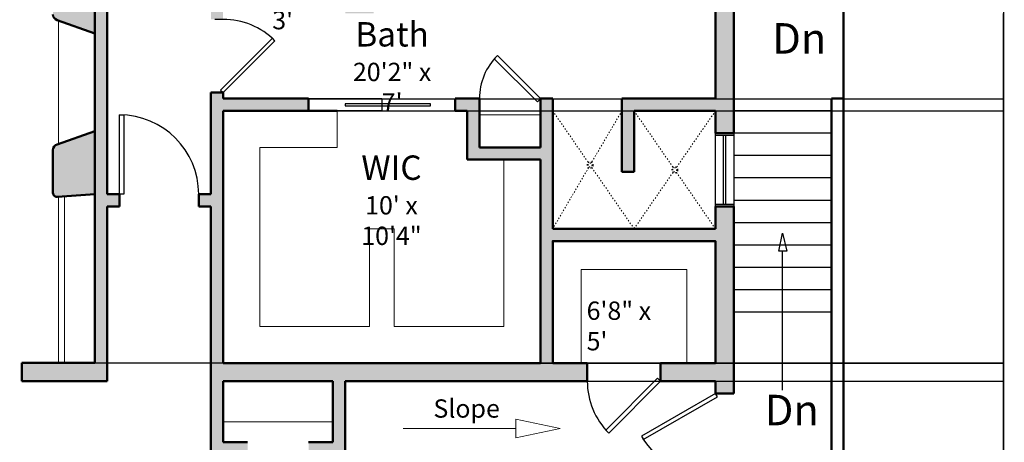
# Model space of a CAD drawing. Units: inches. Extents: x 296 to 2116, y 330 to 1460.
# Tile 4 of 9: x 752 to 1235, y 898 to 1106. Entities that reach past the tile are written whole.
import ezdxf

# ---------------------------------------------------------------- set-up
doc = ezdxf.new("R2010")
doc.units = ezdxf.units.IN
doc.linetypes.add('ACAD_ISO03W100', pattern=[30, 12, -18])
for name, color, linetype, lineweight in [('A-ANNO-DIMS', 2, 'Continuous', 18), ('A-ANNO-SYMB', 2, 'Continuous', 18), ('A-ANNO-TEXT', 7, 'Continuous', 18), ('A-AREA-IDEN', 7, 'Continuous', 25), ('A-DOOR', 3, 'Continuous', 25), ('A-FLOR-FIXT', 8, 'Continuous', 18), ('A-FLOR-OVHD', 132, 'ACAD_ISO03W100', 18), ('A-FLOR-STRS', 40, 'Continuous', 25), ('A-GLAZ', 4, 'Continuous', 25), ('A-WALL', 7, 'Continuous', 50), ('A-WALL-PATT', 8, 'Continuous', 13)]:
    doc.layers.add(name, color=color, linetype=linetype, lineweight=lineweight)
doc.styles.get("Standard").update_dxf_attribs({"font": 'arial.ttf'})
doc.dimstyles.get("Standard").update_dxf_attribs({"dimtxt": 0.18, "dimasz": 0.18, "dimexe": 0.18, "dimexo": 0.0625, "dimgap": 0.09, "dimtad": 0, "dimtih": 1, "dimtoh": 1, "dimdec": 4, "dimzin": 0, "dimdsep": 46, "dimtxsty": 'Standard', "dimcen": 0.09, "dimadec": 0, "dimazin": 0, "dimtfac": 1, "dimtdec": 4, "dimtofl": 0, "dimtmove": 0, "dimatfit": 3, "dimfxl": 1, "dimtolj": 1, "dimtzin": 0, "dimarcsym": 0})

# ---------------------------------------------------------------- blocks, each defined once
blk = doc.blocks.new('*U9')
for p, q in [((0, 0), (0, -4)), ((30, 0), (30, -4))]:
    blk.add_line(p, q)
blk.add_lwpolyline([(0, 0), (21.21, 21.21), (22.45, 19.98), (1.24, -1.24)], close=True)
blk.add_arc((0, 0), 30, 0, 45)
blk = doc.blocks.new('*U11')
for p, q in [((0, 0), (0, -4)), ((-40, 0), (-40, -4))]:
    blk.add_line(p, q)
blk.add_lwpolyline([(0, 0), (-20, 34.64), (-21.52, 33.77), (-1.52, -0.88)], close=True)
blk.add_arc((0, 0), 40, 120, 180)
blk = doc.blocks.new('*U13')
for p, q in [((-32, 0), (-32, 4)), ((0, 0), (0, 4))]:
    blk.add_line(p, q)
blk.add_lwpolyline([(0, 0), (0, -32), (-1.75, -32), (-1.75, 0)], close=True)
blk.add_arc((0, 0), 32, 180, 270)
blk = doc.blocks.new('*U14')
for p, q in [((0, 0), (0, 4)), ((24, 0), (24, 4))]:
    blk.add_line(p, q)
blk.add_lwpolyline([(0, 0), (16.97, -16.97), (18.21, -15.73), (1.24, 1.24)], close=True)
blk.add_arc((0, 0), 24, 315, 0)
blk = doc.blocks.new('*U16')
for p, q in [((0, 0), (0, 4)), ((36, 0), (36, 4))]:
    blk.add_line(p, q)
blk.add_lwpolyline([(0, 0), (25.46, -25.46), (26.69, -24.22), (1.24, 1.24)], close=True)
blk.add_arc((0, 0), 36, 315, 0)
blk = doc.blocks.new('SLOPE-ARROW')
blk.add_line((739.99, 662.71), (684.54, 662.71))
blk.add_lwpolyline([(662.67, 662.71), (684.54, 658.1), (684.54, 667.32)], close=True)
blk = doc.blocks.new('*D45')
at = {"layer": 'A-ANNO-DIMS', "color": 0, "lineweight": -2, "transparency": 16777216}
for p, q in [((1156.58, 1407.95), (1235.3, 1407.95)), ((1235.12, 1407.77), (1235.12, 895.66)), ((1235.12, 383.18), (1235.12, 895.29)), ((609.63, 383), (1235.3, 383))]:
    blk.add_line(p, q, dxfattribs=at)
at = {"layer": 'A-ANNO-DIMS', "color": 0, "transparency": 16777216}
for points in [[(1235.09, 1407.77), (1235.15, 1407.77), (1235.12, 1407.95)], [(1235.09, 383.18), (1235.15, 383.18), (1235.12, 383)]]:
    blk.add_solid(points, dxfattribs=at)
at = {"layer": 'Defpoints', "color": 0, "transparency": 16777216}
for p in [(1156.52, 1407.95), (1235.12, 1407.95), (609.57, 383)]:
    blk.add_point(p, dxfattribs=at)
at = {"layer": 'A-ANNO-DIMS', "color": 0, "transparency": 16777216, "insert": (1235.12, 895.48), "char_height": 0.18, "attachment_point": 5}
blk.add_mtext('\\A1;1025', dxfattribs=at)
blk = doc.blocks.new('*D63')
at = {"layer": 'A-ANNO-DIMS', "color": 0, "lineweight": -2, "transparency": 16777216}
for p, q in [((1102.58, 1156.95), (1235.3, 1156.95)), ((1235.12, 1156.77), (1235.12, 973.64)), ((1235.12, 790.13), (1235.12, 973.27)), ((1063.58, 789.95), (1235.3, 789.95))]:
    blk.add_line(p, q, dxfattribs=at)
at = {"layer": 'A-ANNO-DIMS', "color": 0, "transparency": 16777216}
for points in [[(1235.09, 1156.77), (1235.15, 1156.77), (1235.12, 1156.95)], [(1235.09, 790.13), (1235.15, 790.13), (1235.12, 789.95)]]:
    blk.add_solid(points, dxfattribs=at)
at = {"layer": 'Defpoints', "color": 0, "transparency": 16777216}
for p in [(1102.52, 1156.95), (1235.12, 1156.95), (1063.52, 789.95)]:
    blk.add_point(p, dxfattribs=at)
at = {"layer": 'A-ANNO-DIMS', "color": 0, "transparency": 16777216, "insert": (1235.12, 973.45), "char_height": 0.18, "attachment_point": 5}
blk.add_mtext('\\A1;367', dxfattribs=at)
blk = doc.blocks.new('*D83')
at = {"layer": 'A-ANNO-DIMS', "color": 0, "lineweight": -2, "transparency": 16777216}
for p, q in [((851.58, 1150.95), (1235.3, 1150.95)), ((1235.12, 1150.77), (1235.12, 1109.14)), ((1235.12, 1067.13), (1235.12, 1108.77)), ((851.58, 1066.95), (1235.3, 1066.95))]:
    blk.add_line(p, q, dxfattribs=at)
at = {"layer": 'A-ANNO-DIMS', "color": 0, "transparency": 16777216}
for points in [[(1235.09, 1150.77), (1235.15, 1150.77), (1235.12, 1150.95)], [(1235.09, 1067.13), (1235.15, 1067.13), (1235.12, 1066.95)]]:
    blk.add_solid(points, dxfattribs=at)
at = {"layer": 'Defpoints', "color": 0, "transparency": 16777216}
for p in [(851.52, 1150.95), (1235.12, 1150.95), (851.52, 1066.95)]:
    blk.add_point(p, dxfattribs=at)
at = {"layer": 'A-ANNO-DIMS', "color": 0, "transparency": 16777216, "insert": (1235.12, 1108.95), "char_height": 0.18, "attachment_point": 5}
blk.add_mtext('\\A1;84.00', dxfattribs=at)
blk = doc.blocks.new('*D84')
at = {"layer": 'A-ANNO-DIMS', "color": 0, "lineweight": -2, "transparency": 16777216}
for p, q in [((851.58, 1060.95), (1235.3, 1060.95)), ((1235.12, 1060.77), (1235.12, 999.14)), ((1235.12, 937.13), (1235.12, 998.77)), ((851.58, 936.95), (1235.3, 936.95))]:
    blk.add_line(p, q, dxfattribs=at)
at = {"layer": 'A-ANNO-DIMS', "color": 0, "transparency": 16777216}
for points in [[(1235.09, 1060.77), (1235.15, 1060.77), (1235.12, 1060.95)], [(1235.09, 937.13), (1235.15, 937.13), (1235.12, 936.95)]]:
    blk.add_solid(points, dxfattribs=at)
at = {"layer": 'Defpoints', "color": 0, "transparency": 16777216}
for p in [(851.52, 1060.95), (1235.12, 1060.95), (851.52, 936.95)]:
    blk.add_point(p, dxfattribs=at)
at = {"layer": 'A-ANNO-DIMS', "color": 0, "transparency": 16777216, "insert": (1235.12, 998.95), "char_height": 0.18, "attachment_point": 5}
blk.add_mtext('\\A1;124.00', dxfattribs=at)
blk = doc.blocks.new('*D85')
at = {"layer": 'A-ANNO-DIMS', "color": 0, "lineweight": -2, "transparency": 16777216}
for p, q in [((788.58, 1213), (1235.3, 1213)), ((1235.12, 1212.82), (1235.12, 1075.18)), ((1235.12, 937.18), (1235.12, 1074.82)), ((788.58, 937), (1235.3, 937))]:
    blk.add_line(p, q, dxfattribs=at)
at = {"layer": 'A-ANNO-DIMS', "color": 0, "transparency": 16777216}
for points in [[(1235.09, 1212.82), (1235.15, 1212.82), (1235.12, 1213)], [(1235.09, 937.18), (1235.15, 937.18), (1235.12, 937)]]:
    blk.add_solid(points, dxfattribs=at)
at = {"layer": 'Defpoints', "color": 0, "transparency": 16777216}
for p in [(788.52, 1213), (1235.12, 1213), (788.52, 937)]:
    blk.add_point(p, dxfattribs=at)
at = {"layer": 'A-ANNO-DIMS', "color": 0, "transparency": 16777216, "insert": (1235.12, 1075), "char_height": 0.18, "attachment_point": 5}
blk.add_mtext('\\A1;276.00', dxfattribs=at)
blk = doc.blocks.new('*D98')
at = {"layer": 'A-ANNO-DIMS', "color": 0, "lineweight": -2, "transparency": 16777216}
for p, q in [((1030.58, 927.95), (1235.3, 927.95)), ((1235.12, 927.77), (1235.12, 859.14)), ((1235.12, 790.13), (1235.12, 858.77)), ((1093.58, 789.95), (1235.3, 789.95))]:
    blk.add_line(p, q, dxfattribs=at)
at = {"layer": 'A-ANNO-DIMS', "color": 0, "transparency": 16777216}
for points in [[(1235.09, 927.77), (1235.15, 927.77), (1235.12, 927.95)], [(1235.09, 790.13), (1235.15, 790.13), (1235.12, 789.95)]]:
    blk.add_solid(points, dxfattribs=at)
at = {"layer": 'Defpoints', "color": 0, "transparency": 16777216}
for p in [(1030.52, 927.95), (1235.12, 927.95), (1093.52, 789.95)]:
    blk.add_point(p, dxfattribs=at)
at = {"layer": 'A-ANNO-DIMS', "color": 0, "transparency": 16777216, "insert": (1235.12, 858.95), "char_height": 0.18, "attachment_point": 5}
blk.add_mtext('\\A1;138.00', dxfattribs=at)

msp = doc.modelspace()

# ---------------------------------------------------------------- hatches: boundary and pattern name
at = {"layer": 'A-WALL-PATT'}
h = msp.add_hatch(color=256, dxfattribs=at)
h.dxf.hatch_style = 1
h.paths.add_polyline_path([(656.5723, 927.9991), (668.5723, 927.9991), (668.5723, 936.9991), (650.5723, 936.9991), (650.5723, 897.9991), (356.5223, 897.9991), (356.5223, 955.9991), (347.5223, 955.9991), (347.5223, 888.9991), (423.5723, 888.9991), (423.5723, 766.9991), (432.5723, 766.9991), (432.5723, 834.9991), (453.5723, 834.9991), (468.5723, 834.9991), (468.5723, 840.9991), (432.5723, 840.9991), (432.5723, 888.9991), (504.5723, 888.9991), (504.5723, 840.9991), (504.5723, 834.9991), (531.6223, 834.9991), (531.6223, 768.5344), (527.8443, 764.7564), (530.6728, 761.928), (532.087, 760.5138), (540.5723, 768.9991), (598.0723, 768.9991), (598.0723, 777.9991), (601.8223, 777.9991), (601.8223, 782.1991), (601.8223, 783.9991), (598.0723, 783.9991), (598.0723, 798.9991), (592.0723, 798.9991), (592.0723, 774.9991), (537.6223, 774.9991), (537.6223, 834.9991), (592.0723, 834.9991), (592.0723, 828.9991), (598.0723, 828.9991), (598.0723, 834.9991), (647.5723, 834.9991), (647.5723, 828.9991), (656.5723, 828.9991), (656.5723, 846.9991), (650.5723, 846.9991), (647.5723, 846.9991), (647.5723, 840.9991), (510.5723, 840.9991), (510.5723, 888.9991), (647.5723, 888.9991), (647.5723, 882.9991), (656.5723, 882.9991)])
h.paths.add_polyline_path([(432.5723, 730.9991), (496.5723, 730.9991), (496.5723, 724.9991), (502.5723, 724.9991), (502.5723, 730.9991), (506.6311, 735.058), (502.3885, 739.3006), (500.087, 736.9991), (432.5723, 736.9991), (432.5723, 742.9991), (423.5723, 742.9991), (423.5723, 641.9991), (490.5723, 641.9991), (490.5723, 597.9991), (531.5723, 597.9991), (531.5723, 606.9991), (499.5723, 606.9991), (499.5723, 650.9991), (502.5723, 650.9991), (502.5723, 659.9991), (496.5723, 659.9991), (493.5723, 659.9991), (493.5723, 650.9991), (432.5723, 650.9991)])
h.paths.add_polyline_path([(656.5723, 689.4991), (662.5473, 689.4991), (662.5473, 698.4991), (656.5723, 698.4991), (656.5723, 789.9991), (647.5723, 789.9991), (647.5723, 783.9991), (643.8223, 783.9991), (643.8223, 777.9991), (647.5723, 777.9991), (647.5723, 606.9991), (615.5723, 606.9991), (615.5723, 597.9991), (656.5723, 597.9991)])
h.paths.add_polyline_path([(761.5223, 780.9541), (797.5223, 780.9541), (797.5223, 789.9541), (761.5223, 789.9541), (761.5223, 858.9541), (797.5223, 858.9541), (797.5223, 867.9541), (752.5223, 867.9541), (752.5223, 698.4991), (746.5473, 698.4991), (746.5473, 694.2991), (746.5473, 689.4991), (752.5223, 689.4991), (752.5223, 624.9541), (761.5223, 624.9541)])
h.paths.add_polyline_path([(1102.5223, 795.9541), (1093.5223, 795.9541), (1093.5223, 789.9541), (1063.5223, 789.9541), (881.5223, 789.9541), (881.5223, 837.9541), (911.5223, 837.9541), (911.5223, 849.9541), (907.5223, 849.9541), (905.5223, 849.9541), (905.5223, 843.9541), (845.5223, 843.9541), (845.5223, 834.9541), (849.0223, 834.9541), (851.5223, 834.9541), (851.5223, 837.9541), (875.5223, 837.9541), (875.5223, 789.9541), (851.5223, 789.9541), (851.5223, 792.9541), (845.5223, 792.9541), (845.5223, 789.9541), (833.5223, 789.9541), (833.5223, 785.1541), (833.5223, 780.9541), (1049.5223, 780.9541), (1049.5223, 726.9541), (1053.7223, 726.9541), (1058.5223, 726.9541), (1058.5223, 780.9541), (1102.5223, 780.9541)])
h.paths.add_polyline_path([(761.5223, 588.9541), (752.5223, 588.9541), (752.5223, 564.9541), (761.5223, 564.9541)])
h.paths.add_polyline_path([(809.5223, 480.9541), (761.5223, 480.9541), (761.5223, 528.9541), (752.5223, 528.9541), (752.5223, 471.9541), (809.5223, 471.9541)])
h.paths.add_polyline_path([(1058.5223, 684.9541), (1049.5223, 684.9541), (1049.5223, 480.9541), (1001.5223, 480.9541), (1001.5223, 476.4541), (1001.5223, 471.9541), (1058.5223, 471.9541)])
h.paths.add_polyline_path([(794.5223, 1013.9991), (800.5223, 1013.9991), (800.5223, 1019.9991), (794.5223, 1019.9991), (794.5223, 1296.9541), (785.5223, 1296.9541), (785.5223, 1221.9991), (752.5223, 1221.9991), (752.5223, 1212.9991), (788.5223, 1212.9991), (788.5223, 936.9991), (752.5223, 936.9991), (752.5223, 927.9991), (794.5223, 927.9991)])
h.paths.add_polyline_path([(450.0223, 1191.9991), (398.5223, 1191.9991), (398.5223, 1137.9991), (407.5223, 1137.9991), (407.5223, 1182.9991), (450.0223, 1182.9991)])
h.paths.add_polyline_path([(576.5223, 1212.9991), (612.5223, 1212.9991), (612.5223, 1221.9991), (567.5223, 1221.9991), (567.5223, 1191.9991), (540.0223, 1191.9991), (540.0223, 1182.9991), (576.5223, 1182.9991)])
h.paths.add_polyline_path([(407.5223, 1060.9991), (398.5223, 1060.9991), (398.5223, 1030.9991), (392.5223, 1030.9991), (392.5223, 1021.9991), (407.5223, 1021.9991)])
h.paths.add_polyline_path([(356.5223, 1030.9991), (347.5223, 1030.9991), (347.5223, 1015.9991), (356.5223, 1015.9991), (356.5223, 1021.9991)])
h.paths.add_polyline_path([(788.5223, 1129.9991), (770.0334, 1131.3572, 0.43585667), (767.8869, 1129.3626), (767.8869, 1108.3618, 0.31855172), (769.8942, 1105.5308), (788.5223, 1098.9991)], flags=17)
h.paths.add_polyline_path([(788.5223, 1050.9991), (769.8942, 1044.4674, 0.31855172), (767.8869, 1041.6364), (767.8869, 1020.6356, 0.43585667), (770.0334, 1018.641), (788.5223, 1019.9991)], flags=17)
h.paths.add_polyline_path([(893.5223, 1066.9541), (851.5223, 1066.9541), (851.5223, 1069.9541), (845.5223, 1069.9541), (845.5223, 1019.9991), (839.5223, 1019.9991), (839.5223, 1013.9991), (845.5223, 1013.9991), (845.5223, 891.9541), (863.5223, 891.9541), (863.5223, 897.9541), (851.5223, 897.9541), (851.5223, 927.9541), (905.5223, 927.9541), (905.5223, 897.9541), (893.5223, 897.9541), (893.5223, 891.9541), (905.5223, 891.9541), (905.5223, 885.9541), (911.5223, 885.9541), (911.5223, 927.9541), (1030.5223, 927.9541), (1030.5223, 936.9541), (1013.5223, 936.9541), (1013.5223, 996.9541), (1093.5223, 996.9541), (1093.5223, 936.9541), (1066.5223, 936.9541), (1066.5223, 927.9541), (1093.5223, 927.9541), (1093.5223, 921.9541), (1102.5223, 921.9541), (1102.5223, 1013.9541), (1093.5223, 1013.9541), (1093.5223, 1002.9541), (1013.5223, 1002.9541), (1013.5223, 1060.9541), (1013.5223, 1066.9541), (1007.5223, 1066.9541), (1007.5223, 1042.9541), (977.5223, 1042.9541), (977.5223, 1066.9541), (965.5223, 1066.9541), (965.5223, 1060.9541), (971.5223, 1060.9541), (971.5223, 1036.9541), (1007.5223, 1036.9541), (1007.5223, 936.9541), (851.5223, 936.9541), (851.5223, 1060.9541), (893.5223, 1060.9541)])
h.paths.add_polyline_path([(851.5223, 1150.9541), (919.5223, 1150.9541), (919.5223, 1114.9541), (911.5223, 1114.9541), (911.5223, 1108.9541), (925.5223, 1108.9541), (925.5223, 1150.9541), (1007.5223, 1150.9541), (1007.5223, 1114.9541), (1013.5223, 1114.9541), (1013.5223, 1150.9541), (1046.5223, 1150.9541), (1046.5223, 1159.9541), (1007.5223, 1159.9541), (1007.5223, 1186.9541), (998.5223, 1186.9541), (998.5223, 1156.9541), (845.5223, 1156.9541), (845.5223, 1105.9541), (851.5223, 1105.9541)])
h.paths.add_polyline_path([(1102.5223, 1156.9541), (1102.5223, 1159.9541), (1088.5223, 1159.9541), (1088.5223, 1150.9541), (1093.5223, 1150.9541), (1093.5223, 1147.9541), (1102.5223, 1147.9541)])
h.paths.add_polyline_path([(1102.5223, 1111.9541), (1093.5223, 1111.9541), (1093.5223, 1066.9541), (1047.5223, 1066.9541), (1047.5223, 1030.9541), (1053.5223, 1030.9541), (1053.5223, 1060.9541), (1093.5223, 1060.9541), (1093.5223, 1049.9541), (1102.5223, 1049.9541)])
h.paths.add_polyline_path([(1102.5223, 837.9541), (1093.5223, 837.9541), (1093.5223, 831.9541), (1102.5223, 831.9541)], flags=17)
h.paths.add_polyline_path([(1102.5223, 879.9541), (1093.5223, 879.9541), (1093.5223, 873.9541), (1102.5223, 873.9541)])
h.paths.add_polyline_path([(839.5223, 1353.9541), (785.5223, 1353.9541), (785.5223, 1338.9541), (794.5223, 1338.9541), (794.5223, 1344.9541), (839.5223, 1344.9541)])
h.paths.add_polyline_path([(1007.5223, 1353.9541), (953.5223, 1353.9541), (953.5223, 1344.9541), (998.5223, 1344.9541), (998.5223, 1314.9541), (1007.5223, 1314.9541)])
h.paths.add_polyline_path([(917.5223, 1353.9541), (914.5223, 1353.9541), (914.5223, 1344.9541), (917.5223, 1344.9541)])
h.paths.add_polyline_path([(878.5223, 1353.9541), (875.5223, 1353.9541), (875.5223, 1344.9541), (878.5223, 1344.9541)])
h.paths.add_polyline_path([(1007.5223, 1278.9541), (998.5223, 1278.9541), (998.5223, 1222.9541), (1007.5223, 1222.9541)])
h.paths.add_polyline_path([(407.5223, 1101.9991), (398.5223, 1101.9991), (398.5223, 1096.9991), (407.5223, 1096.9991)])
h.paths.add_polyline_path([(560.5723, 606.9991), (557.5723, 606.9991), (557.5723, 597.9991), (560.5723, 597.9991)])
h.paths.add_polyline_path([(589.5723, 606.9991), (586.5723, 606.9991), (586.5723, 597.9991), (589.5723, 597.9991)])

# ---------------------------------------------------------------- linework, layer by layer
at = {"layer": 'A-DOOR'}
for points in [[(893.5223, 1066.9541), (929.5223, 1066.9541), (929.5223, 1060.9541), (893.5223, 1060.9541)], [(911.5223, 1063.4541), (953.5223, 1063.4541), (953.5223, 1064.4541), (911.5223, 1064.4541)]]:
    msp.add_lwpolyline(points, close=True, dxfattribs=at)
at = {"layer": 'A-FLOR-FIXT'}
for p, q in [((770.5223, 1044.6876), (770.5223, 1105.3105)), ((907.5223, 1042.9541), (907.5223, 1060.9541)), ((1007.5223, 1058.9541), (977.5223, 1058.9541)), ((770.5223, 936.9991), (770.5223, 1018.6769)), ((773.5223, 936.9991), (773.5223, 1018.8972)), ((905.5223, 907.9541), (851.5223, 907.9541))]:
    msp.add_line(p, q, dxfattribs=at)
for points in [[(907.5223, 1042.9541), (869.5223, 1042.9541), (869.5223, 954.9541), (923.5223, 954.9541), (923.5223, 1002.9541), (935.5223, 1002.9541), (935.5223, 954.9541), (989.5223, 954.9541), (989.5223, 1036.9541)], [(1079.5223, 936.9541), (1079.5223, 982.9541), (1027.5223, 982.9541), (1027.5223, 936.9541)]]:
    msp.add_lwpolyline(points, dxfattribs=at)
at = {"layer": 'A-FLOR-OVHD', "ltscale": 0.05}
for p, q in [((1013.5223, 1060.9541), (1031.049, 1035.5403)), ((1047.5223, 1060.9541), (1032.6592, 1035.5995)), ((1053.5223, 1060.9541), (1072.6707, 1033.1889)), ((1093.5223, 1060.9541), (1074.3739, 1033.1889)), ((1031.1421, 1033.0114), (1013.5223, 1002.9541)), ((1032.7522, 1033.0706), (1053.5223, 1002.9541)), ((1072.6707, 1030.7193), (1053.5223, 1002.9541)), ((1074.3739, 1030.7193), (1093.5223, 1002.9541))]:
    msp.add_line(p, q, dxfattribs=at)
msp.add_lwpolyline([(1047.5223, 1060.9541), (1013.5223, 1060.9541), (1013.5223, 1002.9541), (1093.5223, 1002.9541), (1093.5223, 1060.9541), (1053.5223, 1060.9541)], dxfattribs=at)
for centre, radius in [((1031.9006, 1034.3054), 1.5), ((1031.9006, 1034.3054), 1), ((1073.5223, 1031.9541), 1.5), ((1073.5223, 1031.9541), 1)]:
    msp.add_circle(centre, radius, dxfattribs=at)
at = {"layer": 'A-FLOR-STRS'}
for p, q in [((1150.5223, 1060.9541), (1102.5223, 1060.9541)), ((1150.5223, 1049.9541), (1102.5223, 1049.9541)), ((1150.5223, 1038.9541), (1102.5223, 1038.9541)), ((1150.5223, 1027.9541), (1102.5223, 1027.9541)), ((1150.5223, 1016.9541), (1102.5223, 1016.9541)), ((1150.5223, 1005.9541), (1102.5223, 1005.9541)), ((1150.5223, 994.9541), (1102.5223, 994.9541)), ((1150.5223, 983.9541), (1102.5223, 983.9541)), ((1150.5223, 972.9541), (1102.5223, 972.9541)), ((1150.5223, 961.9541), (1102.5223, 961.9541))]:
    msp.add_line(p, q, dxfattribs=at)
msp.add_lwpolyline([(1126.39, 1000.866), (1128.535, 991.9981), (1124.6418, 991.9981)], close=True, dxfattribs=at)
msp.add_lwpolyline([(1126.39, 923.6575), (1126.39, 991.9981)], dxfattribs=at)
at = {"layer": 'A-GLAZ'}
for p, q in [((1093.5223, 1048.9541), (1102.5223, 1048.9541)), ((1097.5223, 1014.9541), (1097.5223, 1048.9541)), ((1098.5223, 1048.9541), (1098.5223, 1014.9541)), ((1102.5223, 1014.9541), (1093.5223, 1014.9541))]:
    msp.add_line(p, q, dxfattribs=at)
msp.add_lwpolyline([(1102.5223, 1013.9541), (1093.5223, 1013.9541), (1093.5223, 1049.9541), (1102.5223, 1049.9541)], close=True, dxfattribs=at)
at = {"layer": 'A-WALL'}
for p, q in [((1156.5223, 576.9541), (1156.5223, 1407.9541)), ((794.5223, 1019.9991), (794.5223, 1296.9541)), ((788.5223, 936.9991), (788.5223, 1212.9991)), ((1093.5223, 1066.9541), (1093.5223, 1111.9541)), ((1102.5223, 1049.9541), (1102.5223, 1111.9541)), ((788.5223, 1098.9991), (769.8942, 1105.5308)), ((851.5223, 1069.9541), (845.5223, 1069.9541)), ((845.5223, 1019.9991), (845.5223, 1069.9541)), ((851.5223, 1066.9541), (851.5223, 1069.9541)), ((893.5223, 1066.9541), (851.5223, 1066.9541)), ((893.5223, 1060.9541), (893.5223, 1066.9541)), ((977.5223, 1066.9541), (965.5223, 1066.9541)), ((965.5223, 1060.9541), (965.5223, 1066.9541)), ((977.5223, 1042.9541), (977.5223, 1066.9541)), ((1007.5223, 1042.9541), (1007.5223, 1066.9541)), ((1013.5223, 1066.9541), (1007.5223, 1066.9541)), ((1013.5223, 1002.9541), (1013.5223, 1066.9541)), ((1093.5223, 1066.9541), (1047.5223, 1066.9541)), ((1047.5223, 1030.9541), (1047.5223, 1066.9541)), ((1150.5223, 576.9541), (1150.5223, 1066.9541)), ((1150.5223, 1066.9541), (1156.5223, 1066.9541)), ((907.5223, 1060.9541), (851.5223, 1060.9541)), ((851.5223, 1060.9541), (851.5223, 936.9541)), ((971.5223, 1060.9541), (965.5223, 1060.9541)), ((971.5223, 1036.9541), (971.5223, 1060.9541)), ((1093.5223, 1060.9541), (1053.5223, 1060.9541)), ((1053.5223, 1060.9541), (1053.5223, 1030.9541)), ((1093.5223, 1049.9541), (1093.5223, 1060.9541)), ((788.5223, 1050.9991), (769.8942, 1044.4674)), ((1093.5223, 1049.9541), (1102.5223, 1049.9541)), ((767.8869, 1041.6364), (767.8869, 1020.6356)), ((1007.5223, 1042.9541), (977.5223, 1042.9541)), ((1007.5223, 1036.9541), (971.5223, 1036.9541)), ((1007.5223, 936.9541), (1007.5223, 1036.9541)), ((1053.5223, 1030.9541), (1047.5223, 1030.9541)), ((788.5223, 1019.9991), (770.0334, 1018.641)), ((794.5223, 1019.9991), (800.5223, 1019.9991)), ((800.5223, 1019.9991), (800.5223, 1013.9991)), ((839.5223, 1019.9991), (839.5223, 1013.9991)), ((839.5223, 1019.9991), (845.5223, 1019.9991)), ((794.5223, 927.9991), (794.5223, 1013.9991)), ((794.5223, 1013.9991), (800.5223, 1013.9991)), ((839.5223, 1013.9991), (845.5223, 1013.9991)), ((845.5223, 891.9541), (845.5223, 1013.9991)), ((1093.5223, 1002.9541), (1093.5223, 1013.9541)), ((1093.5223, 1013.9541), (1102.5223, 1013.9541)), ((1102.5223, 921.9541), (1102.5223, 1013.9541)), ((1093.5223, 1002.9541), (1013.5223, 1002.9541)), ((752.5223, 936.9991), (752.5223, 927.9991)), ((788.5223, 936.9991), (752.5223, 936.9991)), ((851.5223, 936.9541), (1007.5223, 936.9541)), ((1030.5223, 936.9541), (1013.5223, 936.9541)), ((1030.5223, 936.9541), (1030.5223, 927.9541)), ((1093.5223, 936.9541), (1066.5223, 936.9541)), ((1066.5223, 936.9541), (1066.5223, 927.9541)), ((794.5223, 927.9991), (752.5223, 927.9991)), ((851.5223, 897.9541), (851.5223, 927.9541)), ((905.5223, 927.9541), (851.5223, 927.9541)), ((905.5223, 897.9541), (905.5223, 927.9541)), ((911.5223, 885.9541), (911.5223, 927.9541)), ((1030.5223, 927.9541), (911.5223, 927.9541)), ((1093.5223, 927.9541), (1066.5223, 927.9541)), ((1093.5223, 921.9541), (1093.5223, 927.9541)), ((1093.5223, 921.9541), (1102.5223, 921.9541)), ((863.5223, 897.9541), (851.5223, 897.9541)), ((905.5223, 897.9541), (893.5223, 897.9541))]:
    msp.add_line(p, q, dxfattribs=at)
msp.add_lwpolyline([(1093.5223, 936.9541), (1093.5223, 996.9541), (1013.5223, 996.9541), (1013.5223, 936.9541)], dxfattribs=at)
for centre, radius, start, end in [((770.8869, 1108.3618), 3, 180, 250.67747), ((770.8869, 1041.6364), 3, 109.32253, 180), ((769.8869, 1020.6356), 2, 180, 274.201204)]:
    msp.add_arc(centre, radius, start, end, dxfattribs=at)

# ---------------------------------------------------------------- block references
at = {"layer": 'A-ANNO-SYMB', "rotation": 180}
msp.add_blockref('SLOPE-ARROW', (1679.9252, 1567.4896), dxfattribs=at)
at = {"layer": 'A-DOOR', "rotation": 90.00000000000003}
msp.add_blockref('*U16', (851.5223, 1069.9541), dxfattribs=at)
at = {"layer": 'A-DOOR'}
for name, p, xscale, yscale, zscale, rotation in [('*U14', (1007.5223, 1066.9541), 1.250000000000001, 1.250000000000001, 1.250000000000001, 180), ('*U13', (800.5223, 1019.9991), 1.218750000000011, 1.218750000000011, 1.218750000000011, 180), ('*U9', (1066.5223, 927.9541), 1.199999999999999, 1.199999999999999, 1.199999999999999, 180), ('*U11', (1093.5223, 921.9541), 1.05, 1.05, 1.05, 90.00000000000003)]:
    msp.add_blockref(name, p, dxfattribs=dict(at, xscale=xscale, yscale=yscale, zscale=zscale, rotation=rotation))

# ---------------------------------------------------------------- texts
at = {"layer": 'A-ANNO-TEXT'}
for s, width, insert, char_height, attachment_point in [('{\\fArial|b1|i0|c0|p34;Dn}', 22.506546, (1121.4313, 1104.0827), 15, 1), ('\\pxqc;Slope', 41.969454, (992.1912, 919.0734), 9, 3), ('{\\fArial|b1|i0|c0|p34;Dn}', 22.506546, (1117.7618, 921.3076), 15, 1)]:
    msp.add_mtext_dynamic_manual_height_columns(s, width=width, gutter_width=12.5, heights=[0], dxfattribs=dict(at, insert=insert, char_height=char_height, attachment_point=attachment_point))
at = {"layer": 'A-AREA-IDEN', "attachment_point": 1}
for s, width, insert, char_height in [('5\'8" x 3\'', 42.589055, (875.6571, 1125.0707), 9), ('\\pxqc;Bath\\P{\\H0.75x;20\'2" x 7\'}', 49.570994, (909.7915, 1104.6027), 12), ('\\pxqc;WIC\\P{\\H0.75x;10\' x 10\'4"}', 55.821669, (906.3536, 1039.0154), 12), ('6\'8" x 5\'', 43.7979, (1030.1868, 967.1826), 9)]:
    msp.add_mtext_dynamic_manual_height_columns(s, width=width, gutter_width=12.5, heights=[0], dxfattribs=dict(at, insert=insert, char_height=char_height))

# ---------------------------------------------------------------- dimensions: what is measured, and where the dimension line sits
at = {"layer": 'A-ANNO-DIMS'}
for base, p1, p2, override, picture, middle in [((1235.1223, 1407.9541), (609.5723, 382.9991), (1156.5223, 1407.9541), {"dimdec": 0, "dimlfac": 1, "dimrnd": 0, "dimzin": 0, "dimdsep": 46, "dimlunit": 2}, '*D45', (1235.1223, 895.4766)), ((1235.1223, 1212.9991), (788.5223, 936.9991), (788.5223, 1212.9991), {"dimdec": 2, "dimlfac": 1, "dimrnd": 0, "dimzin": 0, "dimdsep": 46, "dimlunit": 2}, '*D85', (1235.1223, 1074.9991)), ((1235.1223, 1156.9541), (1063.5223, 789.9541), (1102.5223, 1156.9541), {"dimdec": 0, "dimlfac": 1, "dimrnd": 0, "dimzin": 0, "dimdsep": 46, "dimlunit": 2}, '*D63', (1235.1223, 973.4541)), ((1235.1223, 1150.9541), (851.5223, 1066.9541), (851.5223, 1150.9541), {"dimdec": 2, "dimlfac": 1, "dimrnd": 0, "dimzin": 0, "dimdsep": 46, "dimlunit": 2}, '*D83', (1235.1223, 1108.9541)), ((1235.1223, 1060.9541), (851.5223, 936.9541), (851.5223, 1060.9541), {"dimdec": 2, "dimlfac": 1, "dimrnd": 0, "dimzin": 0, "dimdsep": 46, "dimlunit": 2}, '*D84', (1235.1223, 998.9541)), ((1235.1223, 927.9541), (1093.5223, 789.9541), (1030.5223, 927.9541), {"dimdec": 2, "dimlfac": 1, "dimrnd": 0, "dimzin": 0, "dimdsep": 46, "dimlunit": 2}, '*D98', (1235.1223, 858.9541))]:
    dim = msp.add_linear_dim(base=base, p1=p1, p2=p2, angle=90, dimstyle='Standard', override=override, dxfattribs=at)
    dim.commit()
    dim.dimension.update_dxf_attribs({"geometry": picture, "text_midpoint": middle})

doc.saveas('drawing.dxf')
